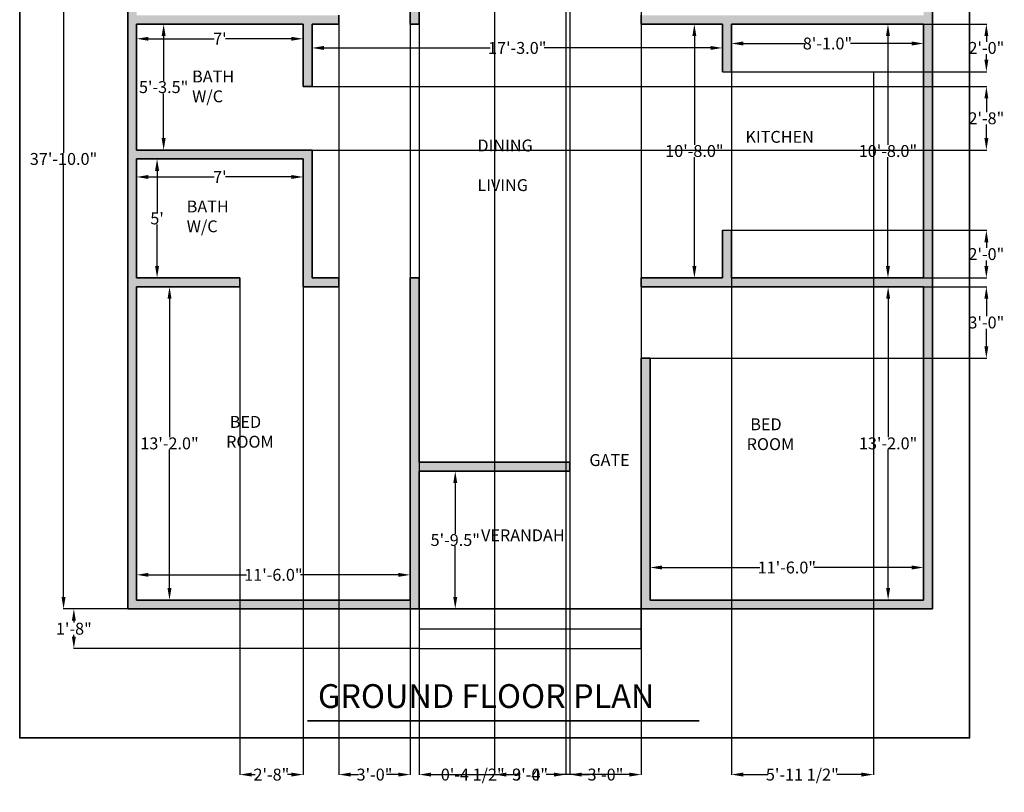
# Model space of a CAD drawing. Units: inches. Extents: x 290 to 786, y 704 to 1301.
# Tile 1 of 2: x 290 to 786, y 704 to 1094. Entities that reach past the tile are written whole.
import ezdxf

# ---------------------------------------------------------------- set-up
doc = ezdxf.new("R2010")
doc.units = ezdxf.units.IN
doc.header["$MEASUREMENT"] = 0
for name, color, linetype, lineweight in [('A-ANNO-DIMS', 2, 'Continuous', 18), ('A-ANNO-TEXT', 7, 'Continuous', 18), ('A-ANNO-TTLB', 7, 'Continuous', 35), ('A-AREA-IDEN', 150, 'Continuous', 25), ('A-FLOR-FIXT', 9, 'Continuous', 25), ('A-FLOR-STRS', 7, 'Continuous', 25), ('A-WALL', 7, 'Continuous', 35)]:
    doc.layers.add(name, color=color, linetype=linetype, lineweight=lineweight)
doc.layers.add('A-WALL-PATT', color=2, linetype='Continuous', lineweight=13, true_color=0xf1eb1f)
doc.styles.get("Standard").update_dxf_attribs({"font": 'arial.ttf'})
doc.dimstyles.get("Standard").update_dxf_attribs({"dimtxt": 6, "dimasz": 6, "dimexe": 0.18, "dimexo": 0.0625, "dimgap": 0.09, "dimtad": 0, "dimtih": 1, "dimtoh": 1, "dimdec": 1, "dimzin": 0, "dimdsep": 46, "dimlunit": 3, "dimtxsty": 'Standard', "dimcen": 0.09, "dimadec": 0, "dimazin": 0, "dimtfac": 1, "dimtdec": 1, "dimtofl": 0, "dimtmove": 0, "dimatfit": 3, "dimfxl": 1, "dimtolj": 1, "dimtzin": 0, "dimarcsym": 0})

# ---------------------------------------------------------------- blocks, each defined once
blk = doc.blocks.new('*D6')
at = {"layer": 'A-ANNO-DIMS', "color": 0, "lineweight": -2, "transparency": 16777216}
for p, q in [((648.53, 1091.27), (648.53, 1081.39)), ((745.53, 1091.27), (745.53, 1081.39)), ((654.53, 1081.57), (685.47, 1081.57)), ((739.53, 1081.57), (708.6, 1081.57))]:
    blk.add_line(p, q, dxfattribs=at)
at = {"layer": 'A-ANNO-DIMS', "color": 0, "transparency": 16777216}
for points in [[(654.53, 1082.57), (654.53, 1080.57), (648.53, 1081.57)], [(739.53, 1082.57), (739.53, 1080.57), (745.53, 1081.57)]]:
    blk.add_solid(points, dxfattribs=at)
at = {"layer": 'Defpoints', "color": 0, "transparency": 16777216}
for p in [(648.53, 1091.33), (745.53, 1091.33), (745.53, 1081.57)]:
    blk.add_point(p, dxfattribs=at)
at = {"layer": 'A-ANNO-DIMS', "color": 0, "transparency": 16777216, "insert": (697.03, 1081.57), "char_height": 6, "attachment_point": 5}
blk.add_mtext('\\A1;8\'-1.0"', dxfattribs=at)
blk = doc.blocks.new('*D7')
at = {"layer": 'A-ANNO-DIMS', "color": 0, "lineweight": -2, "transparency": 16777216}
for p, q in [((745.47, 1091.33), (727.35, 1091.33)), ((727.53, 1085.33), (727.53, 1030.48)), ((727.53, 969.33), (727.53, 1024.18)), ((745.47, 963.33), (727.35, 963.33))]:
    blk.add_line(p, q, dxfattribs=at)
at = {"layer": 'A-ANNO-DIMS', "color": 0, "transparency": 16777216}
for points in [[(726.53, 1085.33), (728.53, 1085.33), (727.53, 1091.33)], [(726.53, 969.33), (728.53, 969.33), (727.53, 963.33)]]:
    blk.add_solid(points, dxfattribs=at)
at = {"layer": 'Defpoints', "color": 0, "transparency": 16777216}
for p in [(745.53, 1091.33), (727.53, 963.33), (745.53, 963.33)]:
    blk.add_point(p, dxfattribs=at)
at = {"layer": 'A-ANNO-DIMS', "color": 0, "transparency": 16777216, "insert": (727.53, 1027.33), "char_height": 6, "attachment_point": 5}
blk.add_mtext('\\A1;10\'-8.0"', dxfattribs=at)
blk = doc.blocks.new('*D8')
at = {"layer": 'A-ANNO-DIMS', "color": 0, "lineweight": -2, "transparency": 16777216}
for p, q in [((607.53, 800.89), (607.53, 817.41)), ((613.53, 817.23), (662.92, 817.23)), ((739.53, 817.23), (690.14, 817.23)), ((745.53, 800.89), (745.53, 817.41))]:
    blk.add_line(p, q, dxfattribs=at)
at = {"layer": 'A-ANNO-DIMS', "color": 0, "transparency": 16777216}
for points in [[(613.53, 818.23), (613.53, 816.23), (607.53, 817.23)], [(739.53, 818.23), (739.53, 816.23), (745.53, 817.23)]]:
    blk.add_solid(points, dxfattribs=at)
at = {"layer": 'Defpoints', "color": 0, "transparency": 16777216}
for p in [(745.53, 817.23), (607.53, 800.83), (745.53, 800.83)]:
    blk.add_point(p, dxfattribs=at)
at = {"layer": 'A-ANNO-DIMS', "color": 0, "transparency": 16777216, "insert": (676.53, 817.23), "char_height": 6, "attachment_point": 5}
blk.add_mtext('\\A1;11\'-6.0"', dxfattribs=at)
blk = doc.blocks.new('*D9')
at = {"layer": 'A-ANNO-DIMS', "color": 0, "lineweight": -2, "transparency": 16777216}
for p, q in [((745.47, 958.83), (727.44, 958.83)), ((727.62, 952.83), (727.62, 882.98)), ((727.62, 806.83), (727.62, 876.67)), ((745.47, 800.83), (727.44, 800.83))]:
    blk.add_line(p, q, dxfattribs=at)
at = {"layer": 'A-ANNO-DIMS', "color": 0, "transparency": 16777216}
for points in [[(726.62, 952.83), (728.62, 952.83), (727.62, 958.83)], [(726.62, 806.83), (728.62, 806.83), (727.62, 800.83)]]:
    blk.add_solid(points, dxfattribs=at)
at = {"layer": 'Defpoints', "color": 0, "transparency": 16777216}
for p in [(745.53, 958.83), (727.62, 800.83), (745.53, 800.83)]:
    blk.add_point(p, dxfattribs=at)
at = {"layer": 'A-ANNO-DIMS', "color": 0, "transparency": 16777216, "insert": (727.62, 879.83), "char_height": 6, "attachment_point": 5}
blk.add_mtext('\\A1;13\'-2.0"', dxfattribs=at)
blk = doc.blocks.new('*D10')
at = {"layer": 'A-ANNO-DIMS', "color": 0, "lineweight": -2, "transparency": 16777216}
for p, q in [((348.6, 958.83), (365.31, 958.83)), ((365.13, 952.83), (365.13, 882.98)), ((365.13, 806.83), (365.13, 876.67)), ((348.6, 800.83), (365.31, 800.83))]:
    blk.add_line(p, q, dxfattribs=at)
at = {"layer": 'A-ANNO-DIMS', "color": 0, "transparency": 16777216}
for points in [[(364.13, 952.83), (366.13, 952.83), (365.13, 958.83)], [(364.13, 806.83), (366.13, 806.83), (365.13, 800.83)]]:
    blk.add_solid(points, dxfattribs=at)
at = {"layer": 'Defpoints', "color": 0, "transparency": 16777216}
for p in [(348.53, 958.83), (348.53, 800.83), (365.13, 800.83)]:
    blk.add_point(p, dxfattribs=at)
at = {"layer": 'A-ANNO-DIMS', "color": 0, "transparency": 16777216, "insert": (365.13, 879.83), "char_height": 6, "attachment_point": 5}
blk.add_mtext('\\A1;13\'-2.0"', dxfattribs=at)
blk = doc.blocks.new('*D11')
at = {"layer": 'A-ANNO-DIMS', "color": 0, "lineweight": -2, "transparency": 16777216}
for p, q in [((348.53, 800.89), (348.53, 813.7)), ((354.53, 813.52), (403.92, 813.52)), ((480.53, 813.52), (431.14, 813.52)), ((486.53, 800.89), (486.53, 813.7))]:
    blk.add_line(p, q, dxfattribs=at)
at = {"layer": 'A-ANNO-DIMS', "color": 0, "transparency": 16777216}
for points in [[(354.53, 814.52), (354.53, 812.52), (348.53, 813.52)], [(480.53, 814.52), (480.53, 812.52), (486.53, 813.52)]]:
    blk.add_solid(points, dxfattribs=at)
at = {"layer": 'Defpoints', "color": 0, "transparency": 16777216}
for p in [(486.53, 813.52), (348.53, 800.83), (486.53, 800.83)]:
    blk.add_point(p, dxfattribs=at)
at = {"layer": 'A-ANNO-DIMS', "color": 0, "transparency": 16777216, "insert": (417.53, 813.52), "char_height": 6, "attachment_point": 5}
blk.add_mtext('\\A1;11\'-6.0"', dxfattribs=at)
blk = doc.blocks.new('*D12')
at = {"layer": 'A-ANNO-DIMS', "color": 0, "lineweight": -2, "transparency": 16777216}
for p, q in [((348.6, 1091.33), (362.35, 1091.33)), ((362.17, 1085.33), (362.17, 1062.73)), ((362.17, 1033.83), (362.17, 1056.42)), ((348.6, 1027.83), (362.35, 1027.83))]:
    blk.add_line(p, q, dxfattribs=at)
at = {"layer": 'A-ANNO-DIMS', "color": 0, "transparency": 16777216}
for points in [[(361.17, 1085.33), (363.17, 1085.33), (362.17, 1091.33)], [(361.17, 1033.83), (363.17, 1033.83), (362.17, 1027.83)]]:
    blk.add_solid(points, dxfattribs=at)
at = {"layer": 'Defpoints', "color": 0, "transparency": 16777216}
for p in [(348.53, 1091.33), (348.53, 1027.83), (362.17, 1027.83)]:
    blk.add_point(p, dxfattribs=at)
at = {"layer": 'A-ANNO-DIMS', "color": 0, "transparency": 16777216, "insert": (362.17, 1059.58), "char_height": 6, "attachment_point": 5}
blk.add_mtext('\\A1;5\'-3.5"', dxfattribs=at)
blk = doc.blocks.new('*D13')
at = {"layer": 'A-ANNO-DIMS', "color": 0, "lineweight": -2, "transparency": 16777216}
for p, q in [((348.53, 1091.27), (348.53, 1083.77)), ((432.53, 1091.27), (432.53, 1083.77)), ((354.53, 1083.95), (387.71, 1083.95)), ((426.53, 1083.95), (393.36, 1083.95))]:
    blk.add_line(p, q, dxfattribs=at)
at = {"layer": 'A-ANNO-DIMS', "color": 0, "transparency": 16777216}
for points in [[(354.53, 1084.95), (354.53, 1082.95), (348.53, 1083.95)], [(426.53, 1084.95), (426.53, 1082.95), (432.53, 1083.95)]]:
    blk.add_solid(points, dxfattribs=at)
at = {"layer": 'Defpoints', "color": 0, "transparency": 16777216}
for p in [(348.53, 1091.33), (432.53, 1091.33), (432.53, 1083.95)]:
    blk.add_point(p, dxfattribs=at)
at = {"layer": 'A-ANNO-DIMS', "color": 0, "transparency": 16777216, "insert": (390.53, 1083.95), "char_height": 6, "attachment_point": 5}
blk.add_mtext("\\A1;7'", dxfattribs=at)
blk = doc.blocks.new('*D14')
at = {"layer": 'A-ANNO-DIMS', "color": 0, "lineweight": -2, "transparency": 16777216}
for p, q in [((348.6, 1023.33), (359.04, 1023.33)), ((358.86, 1017.33), (358.86, 996.47)), ((358.86, 969.33), (358.86, 990.19)), ((348.6, 963.33), (359.04, 963.33))]:
    blk.add_line(p, q, dxfattribs=at)
at = {"layer": 'A-ANNO-DIMS', "color": 0, "transparency": 16777216}
for points in [[(357.86, 1017.33), (359.86, 1017.33), (358.86, 1023.33)], [(357.86, 969.33), (359.86, 969.33), (358.86, 963.33)]]:
    blk.add_solid(points, dxfattribs=at)
at = {"layer": 'Defpoints', "color": 0, "transparency": 16777216}
for p in [(348.53, 1023.33), (358.86, 1023.33), (348.53, 963.33)]:
    blk.add_point(p, dxfattribs=at)
at = {"layer": 'A-ANNO-DIMS', "color": 0, "transparency": 16777216, "insert": (358.86, 993.33), "char_height": 6, "attachment_point": 5}
blk.add_mtext("\\A1;5'", dxfattribs=at)
blk = doc.blocks.new('*D15')
at = {"layer": 'A-ANNO-DIMS', "color": 0, "lineweight": -2, "transparency": 16777216}
for p, q in [((348.53, 1023.27), (348.53, 1014.06)), ((432.53, 1023.27), (432.53, 1014.06)), ((354.53, 1014.24), (387.71, 1014.24)), ((426.53, 1014.24), (393.36, 1014.24))]:
    blk.add_line(p, q, dxfattribs=at)
at = {"layer": 'A-ANNO-DIMS', "color": 0, "transparency": 16777216}
for points in [[(354.53, 1015.24), (354.53, 1013.24), (348.53, 1014.24)], [(426.53, 1015.24), (426.53, 1013.24), (432.53, 1014.24)]]:
    blk.add_solid(points, dxfattribs=at)
at = {"layer": 'Defpoints', "color": 0, "transparency": 16777216}
for p in [(348.53, 1023.33), (432.53, 1023.33), (432.53, 1014.24)]:
    blk.add_point(p, dxfattribs=at)
at = {"layer": 'A-ANNO-DIMS', "color": 0, "transparency": 16777216, "insert": (390.53, 1014.24), "char_height": 6, "attachment_point": 5}
blk.add_mtext("\\A1;7'", dxfattribs=at)
blk = doc.blocks.new('*D16')
at = {"layer": 'A-ANNO-DIMS', "color": 0, "lineweight": -2, "transparency": 16777216}
for p, q in [((491.1, 865.83), (509.45, 865.83)), ((509.27, 859.83), (509.27, 834.23)), ((509.27, 802.33), (509.27, 827.93)), ((491.1, 796.33), (509.45, 796.33))]:
    blk.add_line(p, q, dxfattribs=at)
at = {"layer": 'A-ANNO-DIMS', "color": 0, "transparency": 16777216}
for points in [[(508.27, 859.83), (510.27, 859.83), (509.27, 865.83)], [(508.27, 802.33), (510.27, 802.33), (509.27, 796.33)]]:
    blk.add_solid(points, dxfattribs=at)
at = {"layer": 'Defpoints', "color": 0, "transparency": 16777216}
for p in [(491.03, 865.83), (509.27, 865.83), (491.03, 796.33)]:
    blk.add_point(p, dxfattribs=at)
at = {"layer": 'A-ANNO-DIMS', "color": 0, "transparency": 16777216, "insert": (509.27, 831.08), "char_height": 6, "width": 22.94, "attachment_point": 5}
blk.add_mtext('\\A1;5\'-9.5"', dxfattribs=at)
blk = doc.blocks.new('*D18')
at = {"layer": 'A-ANNO-DIMS', "color": 0, "lineweight": -2, "transparency": 16777216}
for p, q in [((343.97, 1250.33), (311.5, 1250.33)), ((311.68, 1244.33), (311.68, 1026.48)), ((311.68, 802.33), (311.68, 1020.17)), ((343.97, 796.33), (311.5, 796.33))]:
    blk.add_line(p, q, dxfattribs=at)
at = {"layer": 'A-ANNO-DIMS', "color": 0, "transparency": 16777216}
for points in [[(310.68, 1244.33), (312.68, 1244.33), (311.68, 1250.33)], [(310.68, 802.33), (312.68, 802.33), (311.68, 796.33)]]:
    blk.add_solid(points, dxfattribs=at)
at = {"layer": 'Defpoints', "color": 0, "transparency": 16777216}
for p in [(344.03, 1250.33), (311.68, 796.33), (344.03, 796.33)]:
    blk.add_point(p, dxfattribs=at)
at = {"layer": 'A-ANNO-DIMS', "color": 0, "transparency": 16777216, "insert": (311.68, 1023.33), "char_height": 6, "attachment_point": 5}
blk.add_mtext('\\A1;37\'-10.0"', dxfattribs=at)
blk = doc.blocks.new('*D19')
at = {"layer": 'A-ANNO-DIMS', "color": 0, "lineweight": -2, "transparency": 16777216}
for p, q in [((629.96, 1091.33), (630.07, 1091.33)), ((629.89, 1085.33), (629.89, 1030.48)), ((629.89, 969.33), (629.89, 1024.18)), ((629.96, 963.33), (630.07, 963.33))]:
    blk.add_line(p, q, dxfattribs=at)
at = {"layer": 'A-ANNO-DIMS', "color": 0, "transparency": 16777216}
for points in [[(628.89, 1085.33), (630.89, 1085.33), (629.89, 1091.33)], [(628.89, 969.33), (630.89, 969.33), (629.89, 963.33)]]:
    blk.add_solid(points, dxfattribs=at)
at = {"layer": 'Defpoints', "color": 0, "transparency": 16777216}
for p in [(629.89, 1091.33), (629.89, 963.33), (629.89, 963.33)]:
    blk.add_point(p, dxfattribs=at)
at = {"layer": 'A-ANNO-DIMS', "color": 0, "transparency": 16777216, "insert": (629.89, 1027.33), "char_height": 6, "attachment_point": 5}
blk.add_mtext('\\A1;10\'-8.0"', dxfattribs=at)
blk = doc.blocks.new('*D20')
at = {"layer": 'A-ANNO-DIMS', "color": 0, "lineweight": -2, "transparency": 16777216}
for p, q in [((437.03, 1091.27), (437.03, 1079.15)), ((644.03, 1091.27), (644.03, 1079.15)), ((443.03, 1079.33), (526.92, 1079.33)), ((638.03, 1079.33), (554.14, 1079.33))]:
    blk.add_line(p, q, dxfattribs=at)
at = {"layer": 'A-ANNO-DIMS', "color": 0, "transparency": 16777216}
for points in [[(443.03, 1080.33), (443.03, 1078.33), (437.03, 1079.33)], [(638.03, 1080.33), (638.03, 1078.33), (644.03, 1079.33)]]:
    blk.add_solid(points, dxfattribs=at)
at = {"layer": 'Defpoints', "color": 0, "transparency": 16777216}
for p in [(437.03, 1091.33), (644.03, 1091.33), (644.03, 1079.33)]:
    blk.add_point(p, dxfattribs=at)
at = {"layer": 'A-ANNO-DIMS', "color": 0, "transparency": 16777216, "insert": (540.53, 1079.33), "char_height": 6, "attachment_point": 5}
blk.add_mtext('\\A1;17\'-3.0"', dxfattribs=at)
blk = doc.blocks.new('*D22')
at = {"layer": 'A-ANNO-DIMS', "color": 0, "lineweight": -2, "transparency": 16777216}
for p, q in [((567.03, 1149.77), (567.03, 712.58)), ((603.03, 1149.77), (603.03, 712.58)), ((573.03, 712.76), (576.97, 712.76)), ((597.03, 712.76), (593.1, 712.76))]:
    blk.add_line(p, q, dxfattribs=at)
at = {"layer": 'A-ANNO-DIMS', "color": 0, "transparency": 16777216}
for points in [[(573.03, 713.76), (573.03, 711.76), (567.03, 712.76)], [(597.03, 713.76), (597.03, 711.76), (603.03, 712.76)]]:
    blk.add_solid(points, dxfattribs=at)
at = {"layer": 'Defpoints', "color": 0, "transparency": 16777216}
for p in [(567.03, 1149.83), (603.03, 1149.83), (603.03, 712.76)]:
    blk.add_point(p, dxfattribs=at)
at = {"layer": 'A-ANNO-DIMS', "color": 0, "transparency": 16777216, "insert": (585.03, 712.76), "char_height": 6, "attachment_point": 5}
blk.add_mtext('\\A1;3\'-0"', dxfattribs=at)
blk = doc.blocks.new('*D24')
at = {"layer": 'A-ANNO-DIMS', "color": 0, "lineweight": -2, "transparency": 16777216}
for p, q in [((529.03, 1149.77), (529.03, 712.58)), ((565.03, 1149.77), (565.03, 712.58)), ((535.03, 712.76), (538.97, 712.76)), ((559.03, 712.76), (555.1, 712.76))]:
    blk.add_line(p, q, dxfattribs=at)
at = {"layer": 'A-ANNO-DIMS', "color": 0, "transparency": 16777216}
for points in [[(535.03, 713.76), (535.03, 711.76), (529.03, 712.76)], [(559.03, 713.76), (559.03, 711.76), (565.03, 712.76)]]:
    blk.add_solid(points, dxfattribs=at)
at = {"layer": 'Defpoints', "color": 0, "transparency": 16777216}
for p in [(529.03, 1149.83), (565.03, 1149.83), (565.03, 712.76)]:
    blk.add_point(p, dxfattribs=at)
at = {"layer": 'A-ANNO-DIMS', "color": 0, "transparency": 16777216, "insert": (547.03, 712.76), "char_height": 6, "attachment_point": 5}
blk.add_mtext('\\A1;3\'-0"', dxfattribs=at)
blk = doc.blocks.new('*D26')
at = {"layer": 'A-ANNO-DIMS', "color": 0, "lineweight": -2, "transparency": 16777216}
for p, q in [((491.03, 776.27), (491.03, 712.58)), ((603.03, 776.27), (603.03, 712.58)), ((497.03, 712.76), (538.97, 712.76)), ((597.03, 712.76), (555.1, 712.76))]:
    blk.add_line(p, q, dxfattribs=at)
at = {"layer": 'A-ANNO-DIMS', "color": 0, "transparency": 16777216}
for points in [[(497.03, 713.76), (497.03, 711.76), (491.03, 712.76)], [(597.03, 713.76), (597.03, 711.76), (603.03, 712.76)]]:
    blk.add_solid(points, dxfattribs=at)
at = {"layer": 'Defpoints', "color": 0, "transparency": 16777216}
for p in [(491.03, 776.33), (603.03, 776.33), (603.03, 712.76)]:
    blk.add_point(p, dxfattribs=at)
at = {"layer": 'A-ANNO-DIMS', "color": 0, "transparency": 16777216, "insert": (547.03, 712.76), "char_height": 6, "attachment_point": 5}
blk.add_mtext('\\A1;9\'-4"', dxfattribs=at)
blk = doc.blocks.new('*D27')
at = {"layer": 'A-ANNO-DIMS', "color": 0, "lineweight": -2, "transparency": 16777216}
for p, q in [((490.97, 796.33), (316.7, 796.33)), ((316.88, 790.33), (316.88, 789.48)), ((316.88, 782.33), (316.88, 783.18)), ((490.97, 776.33), (316.7, 776.33))]:
    blk.add_line(p, q, dxfattribs=at)
at = {"layer": 'A-ANNO-DIMS', "color": 0, "transparency": 16777216}
for points in [[(315.88, 790.33), (317.88, 790.33), (316.88, 796.33)], [(315.88, 782.33), (317.88, 782.33), (316.88, 776.33)]]:
    blk.add_solid(points, dxfattribs=at)
at = {"layer": 'Defpoints', "color": 0, "transparency": 16777216}
for p in [(316.88, 796.33), (491.03, 796.33), (491.03, 776.33)]:
    blk.add_point(p, dxfattribs=at)
at = {"layer": 'A-ANNO-DIMS', "color": 0, "transparency": 16777216, "insert": (316.88, 786.33), "char_height": 6, "attachment_point": 5}
blk.add_mtext('\\A1;1\'-8"', dxfattribs=at)
blk = doc.blocks.new('*D28')
at = {"layer": 'A-ANNO-DIMS', "color": 0, "lineweight": -2, "transparency": 16777216}
for p, q in [((603.03, 922.77), (603.03, 712.58)), ((567.03, 865.77), (567.03, 712.58)), ((573.03, 712.76), (576.97, 712.76)), ((597.03, 712.76), (593.1, 712.76))]:
    blk.add_line(p, q, dxfattribs=at)
at = {"layer": 'A-ANNO-DIMS', "color": 0, "transparency": 16777216}
for points in [[(573.03, 713.76), (573.03, 711.76), (567.03, 712.76)], [(597.03, 713.76), (597.03, 711.76), (603.03, 712.76)]]:
    blk.add_solid(points, dxfattribs=at)
at = {"layer": 'Defpoints', "color": 0, "transparency": 16777216}
for p in [(603.03, 922.83), (567.03, 865.83), (603.03, 712.76)]:
    blk.add_point(p, dxfattribs=at)
at = {"layer": 'A-ANNO-DIMS', "color": 0, "transparency": 16777216, "insert": (585.03, 712.76), "char_height": 6, "attachment_point": 5}
blk.add_mtext('\\A1;3\'-0"', dxfattribs=at)
blk = doc.blocks.new('*D29')
at = {"layer": 'A-ANNO-DIMS', "color": 0, "lineweight": -2, "transparency": 16777216}
for p, q in [((400.53, 958.77), (400.53, 712.58)), ((432.53, 958.77), (432.53, 712.58)), ((406.53, 712.76), (408.42, 712.76)), ((426.53, 712.76), (424.65, 712.76))]:
    blk.add_line(p, q, dxfattribs=at)
at = {"layer": 'A-ANNO-DIMS', "color": 0, "transparency": 16777216}
for points in [[(406.53, 713.76), (406.53, 711.76), (400.53, 712.76)], [(426.53, 713.76), (426.53, 711.76), (432.53, 712.76)]]:
    blk.add_solid(points, dxfattribs=at)
at = {"layer": 'Defpoints', "color": 0, "transparency": 16777216}
for p in [(400.53, 958.83), (432.53, 958.83), (432.53, 712.76)]:
    blk.add_point(p, dxfattribs=at)
at = {"layer": 'A-ANNO-DIMS', "color": 0, "transparency": 16777216, "insert": (416.53, 712.76), "char_height": 6, "attachment_point": 5}
blk.add_mtext('\\A1;2\'-8"', dxfattribs=at)
blk = doc.blocks.new('*D30')
at = {"layer": 'A-ANNO-DIMS', "color": 0, "lineweight": -2, "transparency": 16777216}
for p, q in [((437.1, 1059.83), (777.36, 1059.83)), ((777.18, 1053.83), (777.18, 1046.98)), ((777.18, 1033.83), (777.18, 1040.68)), ((437.1, 1027.83), (777.36, 1027.83))]:
    blk.add_line(p, q, dxfattribs=at)
at = {"layer": 'A-ANNO-DIMS', "color": 0, "transparency": 16777216}
for points in [[(776.18, 1053.83), (778.18, 1053.83), (777.18, 1059.83)], [(776.18, 1033.83), (778.18, 1033.83), (777.18, 1027.83)]]:
    blk.add_solid(points, dxfattribs=at)
at = {"layer": 'Defpoints', "color": 0, "transparency": 16777216}
for p in [(437.03, 1059.83), (777.18, 1059.83), (437.03, 1027.83)]:
    blk.add_point(p, dxfattribs=at)
at = {"layer": 'A-ANNO-DIMS', "color": 0, "transparency": 16777216, "insert": (777.18, 1043.83), "char_height": 6, "attachment_point": 5}
blk.add_mtext('\\A1;2\'-8"', dxfattribs=at)
blk = doc.blocks.new('*D31')
at = {"layer": 'A-ANNO-DIMS', "color": 0, "lineweight": -2, "transparency": 16777216}
for p, q in [((450.53, 958.77), (450.53, 712.58)), ((486.53, 963.27), (486.53, 712.58)), ((456.53, 712.76), (460.47, 712.76)), ((480.53, 712.76), (476.6, 712.76))]:
    blk.add_line(p, q, dxfattribs=at)
at = {"layer": 'A-ANNO-DIMS', "color": 0, "transparency": 16777216}
for points in [[(456.53, 713.76), (456.53, 711.76), (450.53, 712.76)], [(480.53, 713.76), (480.53, 711.76), (486.53, 712.76)]]:
    blk.add_solid(points, dxfattribs=at)
at = {"layer": 'Defpoints', "color": 0, "transparency": 16777216}
for p in [(450.53, 958.83), (486.53, 963.33), (486.53, 712.76)]:
    blk.add_point(p, dxfattribs=at)
at = {"layer": 'A-ANNO-DIMS', "color": 0, "transparency": 16777216, "insert": (468.53, 712.76), "char_height": 6, "attachment_point": 5}
blk.add_mtext('\\A1;3\'-0"', dxfattribs=at)
blk = doc.blocks.new('*D32')
at = {"layer": 'A-ANNO-DIMS', "color": 0, "lineweight": -2, "transparency": 16777216}
for p, q in [((603.1, 958.83), (777.36, 958.83)), ((777.18, 952.83), (777.18, 943.98)), ((777.18, 928.83), (777.18, 937.67)), ((607.6, 922.83), (777.36, 922.83))]:
    blk.add_line(p, q, dxfattribs=at)
at = {"layer": 'A-ANNO-DIMS', "color": 0, "transparency": 16777216}
for points in [[(776.18, 952.83), (778.18, 952.83), (777.18, 958.83)], [(776.18, 928.83), (778.18, 928.83), (777.18, 922.83)]]:
    blk.add_solid(points, dxfattribs=at)
at = {"layer": 'Defpoints', "color": 0, "transparency": 16777216}
for p in [(603.03, 958.83), (607.53, 922.83), (777.18, 922.83)]:
    blk.add_point(p, dxfattribs=at)
at = {"layer": 'A-ANNO-DIMS', "color": 0, "transparency": 16777216, "insert": (777.18, 940.83), "char_height": 6, "attachment_point": 5}
blk.add_mtext('\\A1;3\'-0"', dxfattribs=at)
blk = doc.blocks.new('*D33')
at = {"layer": 'A-ANNO-DIMS', "color": 0, "lineweight": -2, "transparency": 16777216}
for p, q in [((450.53, 1091.27), (450.53, 712.58)), ((486.53, 1091.27), (486.53, 712.58)), ((456.53, 712.76), (460.47, 712.76)), ((480.53, 712.76), (476.6, 712.76))]:
    blk.add_line(p, q, dxfattribs=at)
at = {"layer": 'A-ANNO-DIMS', "color": 0, "transparency": 16777216}
for points in [[(456.53, 713.76), (456.53, 711.76), (450.53, 712.76)], [(480.53, 713.76), (480.53, 711.76), (486.53, 712.76)]]:
    blk.add_solid(points, dxfattribs=at)
at = {"layer": 'Defpoints', "color": 0, "transparency": 16777216}
for p in [(450.53, 1091.33), (486.53, 1091.33), (486.53, 712.76)]:
    blk.add_point(p, dxfattribs=at)
at = {"layer": 'A-ANNO-DIMS', "color": 0, "transparency": 16777216, "insert": (468.53, 712.76), "char_height": 6, "attachment_point": 5}
blk.add_mtext('\\A1;3\'-0"', dxfattribs=at)
blk = doc.blocks.new('*D35')
at = {"layer": 'A-ANNO-DIMS', "color": 0, "lineweight": -2, "transparency": 16777216}
for p, q in [((648.6, 1091.33), (777.36, 1091.33)), ((777.18, 1085.33), (777.18, 1082.48)), ((777.18, 1073.33), (777.18, 1076.18)), ((648.6, 1067.33), (777.36, 1067.33))]:
    blk.add_line(p, q, dxfattribs=at)
at = {"layer": 'A-ANNO-DIMS', "color": 0, "transparency": 16777216}
for points in [[(776.18, 1085.33), (778.18, 1085.33), (777.18, 1091.33)], [(776.18, 1073.33), (778.18, 1073.33), (777.18, 1067.33)]]:
    blk.add_solid(points, dxfattribs=at)
at = {"layer": 'Defpoints', "color": 0, "transparency": 16777216}
for p in [(648.53, 1091.33), (648.53, 1067.33), (777.18, 1067.33)]:
    blk.add_point(p, dxfattribs=at)
at = {"layer": 'A-ANNO-DIMS', "color": 0, "transparency": 16777216, "insert": (777.18, 1079.33), "char_height": 6, "attachment_point": 5}
blk.add_mtext('\\A1;2\'-0"', dxfattribs=at)
blk = doc.blocks.new('*D36')
at = {"layer": 'A-ANNO-DIMS', "color": 0, "lineweight": -2, "transparency": 16777216}
for p, q in [((648.53, 1067.27), (648.53, 712.58)), ((720.17, 1067.27), (720.17, 712.58)), ((654.53, 712.76), (666.97, 712.76)), ((714.17, 712.76), (701.74, 712.76))]:
    blk.add_line(p, q, dxfattribs=at)
at = {"layer": 'A-ANNO-DIMS', "color": 0, "transparency": 16777216}
for points in [[(654.53, 713.76), (654.53, 711.76), (648.53, 712.76)], [(714.17, 713.76), (714.17, 711.76), (720.17, 712.76)]]:
    blk.add_solid(points, dxfattribs=at)
at = {"layer": 'Defpoints', "color": 0, "transparency": 16777216}
for p in [(648.53, 1067.33), (720.17, 1067.33), (720.17, 712.76)]:
    blk.add_point(p, dxfattribs=at)
at = {"layer": 'A-ANNO-DIMS', "color": 0, "transparency": 16777216, "insert": (684.35, 712.76), "char_height": 6, "attachment_point": 5}
blk.add_mtext('\\A1;5\'-11 1/2"', dxfattribs=at)
blk = doc.blocks.new('*D37')
at = {"layer": 'A-ANNO-DIMS', "color": 0, "lineweight": -2, "transparency": 16777216}
for p, q in [((648.6, 987.33), (777.36, 987.33)), ((777.18, 981.33), (777.18, 978.48)), ((777.18, 969.33), (777.18, 972.18)), ((648.6, 963.33), (777.36, 963.33))]:
    blk.add_line(p, q, dxfattribs=at)
at = {"layer": 'A-ANNO-DIMS', "color": 0, "transparency": 16777216}
for points in [[(776.18, 981.33), (778.18, 981.33), (777.18, 987.33)], [(776.18, 969.33), (778.18, 969.33), (777.18, 963.33)]]:
    blk.add_solid(points, dxfattribs=at)
at = {"layer": 'Defpoints', "color": 0, "transparency": 16777216}
for p in [(648.53, 987.33), (777.18, 987.33), (648.53, 963.33)]:
    blk.add_point(p, dxfattribs=at)
at = {"layer": 'A-ANNO-DIMS', "color": 0, "transparency": 16777216, "insert": (777.18, 975.33), "char_height": 6, "attachment_point": 5}
blk.add_mtext('\\A1;2\'-0"', dxfattribs=at)
blk = doc.blocks.new('*D38')
at = {"layer": 'A-ANNO-DIMS', "color": 0, "lineweight": -2, "transparency": 16777216}
for p, q in [((486.53, 1091.27), (486.53, 712.58)), ((491.03, 1091.27), (491.03, 712.58)), ((480.53, 712.76), (474.53, 712.76)), ((497.03, 712.76), (503.03, 712.76))]:
    blk.add_line(p, q, dxfattribs=at)
at = {"layer": 'A-ANNO-DIMS', "color": 0, "transparency": 16777216}
for points in [[(480.53, 713.76), (480.53, 711.76), (486.53, 712.76)], [(497.03, 713.76), (497.03, 711.76), (491.03, 712.76)]]:
    blk.add_solid(points, dxfattribs=at)
at = {"layer": 'Defpoints', "color": 0, "transparency": 16777216}
for p in [(486.53, 1091.33), (491.03, 1091.33), (491.03, 712.76)]:
    blk.add_point(p, dxfattribs=at)
at = {"layer": 'A-ANNO-DIMS', "color": 0, "transparency": 16777216, "insert": (518.09, 712.76), "char_height": 6, "attachment_point": 5}
blk.add_mtext('\\A1;0\'-4 1/2"', dxfattribs=at)

msp = doc.modelspace()

# ---------------------------------------------------------------- hatches: boundary and pattern name
at = {"layer": 'A-WALL-PATT'}
h = msp.add_hatch(color=256, dxfattribs=at)
h.dxf.hatch_style = 1
h.paths.add_polyline_path([(750.03, 1250.33), (344.03, 1250.33), (344.03, 796.33), (491.03, 796.33), (491.03, 865.83), (567.03, 865.83), (567.03, 870.33), (491.03, 870.33), (491.03, 963.33), (486.53, 963.33), (486.53, 800.83), (348.53, 800.83), (348.53, 958.83), (400.53, 958.83), (400.53, 963.33), (348.53, 963.33), (348.53, 1023.33), (432.53, 1023.33), (432.53, 958.83), (450.53, 958.83), (450.53, 963.33), (437.03, 963.33), (437.03, 1027.83), (348.53, 1027.83), (348.53, 1091.33), (432.53, 1091.33), (432.53, 1059.83), (437.03, 1059.83), (437.03, 1091.33), (450.53, 1091.33), (450.53, 1095.83), (348.53, 1095.83), (348.53, 1245.83), (486.53, 1245.83), (486.53, 1091.33), (491.03, 1091.33), (491.03, 1245.83), (603.03, 1245.83), (603.03, 1131.83), (607.53, 1131.83), (607.53, 1245.83), (745.53, 1245.83), (745.53, 1095.83), (603.03, 1095.83), (603.03, 1091.33), (644.03, 1091.33), (644.03, 1067.33), (648.53, 1067.33), (648.53, 1091.33), (745.53, 1091.33), (745.53, 963.33), (648.53, 963.33), (648.53, 987.33), (644.03, 987.33), (644.03, 963.33), (603.03, 963.33), (603.03, 958.83), (745.53, 958.83), (745.53, 800.83), (607.53, 800.83), (607.53, 922.83), (603.03, 922.83), (603.03, 796.33), (750.03, 796.33)])

# ---------------------------------------------------------------- linework, layer by layer
at = {"layer": 'A-ANNO-TTLB'}
for p, q in [((434.67, 739.91), (627.58, 739.91)), ((627.58, 739.91), (632.31, 739.91))]:
    msp.add_line(p, q, dxfattribs=at)
msp.add_lwpolyline([(289.56, 1300.6), (768.7, 1300.6), (768.7, 731.29), (289.56, 731.29)], close=True, dxfattribs=at)
at = {"layer": 'A-FLOR-FIXT'}
for p, q in [((644.03, 1067.33), (720.17, 1067.33)), ((720.17, 1067.33), (720.17, 987.33)), ((644.03, 987.33), (720.17, 987.33))]:
    msp.add_line(p, q, dxfattribs=at)
at = {"layer": 'A-FLOR-STRS'}
for p, q in [((491.03, 796.33), (491.03, 776.33)), ((603.03, 776.33), (603.03, 796.33)), ((491.03, 786.33), (603.03, 786.33)), ((491.03, 776.33), (603.03, 776.33))]:
    msp.add_line(p, q, dxfattribs=at)
at = {"layer": 'A-WALL'}
for p, q in [((344.03, 1250.33), (344.03, 796.33)), ((750.03, 1250.33), (750.03, 796.33)), ((486.53, 1245.83), (486.53, 1091.33)), ((491.03, 1245.83), (491.03, 1091.33)), ((450.53, 1091.33), (450.53, 1095.83)), ((603.03, 1095.83), (603.03, 1091.33)), ((348.53, 1091.33), (432.53, 1091.33)), ((348.53, 1091.33), (348.53, 1027.83)), ((432.53, 1091.33), (432.53, 1059.83)), ((437.03, 1091.33), (437.03, 1059.83)), ((437.03, 1091.33), (450.53, 1091.33)), ((486.53, 1091.33), (491.03, 1091.33)), ((603.03, 1091.33), (644.03, 1091.33)), ((644.03, 1091.33), (644.03, 1067.33)), ((648.53, 1091.33), (648.53, 1067.33)), ((648.53, 1091.33), (648.53, 1067.33)), ((648.53, 1091.33), (745.53, 1091.33)), ((745.53, 1091.33), (745.53, 963.33)), ((432.53, 1059.83), (437.03, 1059.83)), ((348.53, 1027.83), (437.03, 1027.83)), ((348.53, 1023.33), (432.53, 1023.33)), ((348.53, 1023.33), (348.53, 963.33)), ((432.53, 1023.33), (432.53, 958.83)), ((437.03, 1027.83), (437.03, 963.33)), ((644.03, 987.33), (644.03, 963.33)), ((648.53, 963.33), (648.53, 987.33)), ((648.53, 987.33), (648.53, 963.33)), ((348.53, 963.33), (400.53, 963.33)), ((348.53, 958.83), (400.53, 958.83)), ((348.53, 958.83), (348.53, 800.83)), ((400.53, 963.33), (400.53, 958.83)), ((432.53, 958.83), (450.53, 958.83)), ((437.03, 963.33), (450.53, 963.33)), ((450.53, 963.33), (450.53, 958.83)), ((486.53, 963.33), (486.53, 800.83)), ((486.53, 963.33), (491.03, 963.33)), ((491.03, 963.33), (491.03, 870.33)), ((603.03, 963.33), (644.03, 963.33)), ((603.03, 963.33), (603.03, 958.83)), ((603.03, 958.83), (745.53, 958.83)), ((648.53, 963.33), (745.53, 963.33)), ((745.53, 958.83), (745.53, 800.83)), ((603.03, 922.83), (607.53, 922.83)), ((603.03, 922.83), (603.03, 796.33)), ((607.53, 922.83), (607.53, 800.83)), ((491.03, 870.33), (567.03, 870.33)), ((567.03, 865.83), (567.03, 870.33)), ((491.03, 865.83), (567.03, 865.83)), ((491.03, 865.83), (491.03, 796.33)), ((348.53, 800.83), (486.53, 800.83)), ((607.53, 800.83), (745.53, 800.83)), ((344.03, 796.33), (750.03, 796.33))]:
    msp.add_line(p, q, dxfattribs=at)

# ---------------------------------------------------------------- texts
at = {"layer": 'A-ANNO-TEXT', "insert": (576.93, 874.42), "char_height": 6, "attachment_point": 1}
msp.add_mtext_dynamic_manual_height_columns('GATE', width=21.2425, gutter_width=30, heights=[0], dxfattribs=at)
at = {"layer": 'A-ANNO-TTLB', "insert": (440, 758.37), "char_height": 12, "attachment_point": 1}
msp.add_mtext_dynamic_manual_height_columns('GROUND FLOOR PLAN', width=230.1331, gutter_width=60, heights=[0], dxfattribs=at)
at = {"layer": 'A-AREA-IDEN', "char_height": 6, "attachment_point": 1}
for s, width, insert in [('BATH\\PW/C', 49.7176, (376.53, 1067.92)), ('DINING\\P\\PLIVING', 66.1278, (520.44, 1033.13)), ('KITCHEN', 49.9801, (655.65, 1037.48)), ('BATH\\PW/C', 33.3903, (373.8, 1002.34)), (' BED\\PROOM', 38.2318, (393.69, 893.68)), (' BED\\PROOM', 42.9072, (656.26, 892.46)), ('VERANDAH', 36.2763, (522.28, 836.45))]:
    msp.add_mtext_dynamic_manual_height_columns(s, width=width, gutter_width=30, heights=[0], dxfattribs=dict(at, insert=insert))

# ---------------------------------------------------------------- dimensions: what is measured, and where the dimension line sits
at = {"layer": 'A-ANNO-DIMS'}
for base, p1, p2, override, picture, middle in [((311.68, 796.33), (344.03, 1250.33), (344.03, 796.33), {"dimclrd": 0, "dimclre": 0, "dimclrt": 0}, '*D18', (311.68, 1023.33)), ((362.17, 1027.83), (348.53, 1091.33), (348.53, 1027.83), {"dimclrd": 0, "dimclre": 0, "dimclrt": 0}, '*D12', (362.17, 1059.58)), ((629.89, 963.33), (629.89, 1091.33), (629.89, 963.33), {"dimclrd": 0, "dimclre": 0, "dimclrt": 0}, '*D19', (629.89, 1027.33)), ((777.18, 1067.33), (648.53, 1091.33), (648.53, 1067.33), {"dimdec": 1, "dimlfac": 1, "dimrnd": 0, "dimzin": 1, "dimdsep": 46, "dimlunit": 4, "dimfrac": 2}, '*D35', (777.18, 1079.33)), ((727.53, 963.33), (745.53, 1091.33), (745.53, 963.33), {"dimclrd": 0, "dimclre": 0, "dimclrt": 0}, '*D7', (727.53, 1027.33)), ((777.18, 1059.83), (437.03, 1027.83), (437.03, 1059.83), {"dimdec": 1, "dimlfac": 1, "dimrnd": 0, "dimzin": 1, "dimdsep": 46, "dimlunit": 4, "dimfrac": 2}, '*D30', (777.18, 1043.83)), ((358.86, 1023.33), (348.53, 963.33), (348.53, 1023.33), {"dimclrd": 0, "dimclre": 0, "dimclrt": 0}, '*D14', (358.86, 993.33)), ((777.18, 987.33), (648.53, 963.33), (648.53, 987.33), {"dimdec": 1, "dimlfac": 1, "dimrnd": 0, "dimzin": 1, "dimdsep": 46, "dimlunit": 4, "dimfrac": 2}, '*D37', (777.18, 975.33)), ((365.13, 800.83), (348.53, 958.83), (348.53, 800.83), {"dimclrd": 0, "dimclre": 0, "dimclrt": 0}, '*D10', (365.13, 879.83)), ((777.18, 922.83), (603.03, 958.83), (607.53, 922.83), {"dimdec": 1, "dimlfac": 1, "dimrnd": 0, "dimzin": 1, "dimdsep": 46, "dimlunit": 4, "dimfrac": 2}, '*D32', (777.18, 940.83)), ((727.62, 800.83), (745.53, 958.83), (745.53, 800.83), {"dimclrd": 0, "dimclre": 0, "dimclrt": 0}, '*D9', (727.62, 879.83)), ((509.27, 865.83), (491.03, 796.33), (491.03, 865.83), {"dimclrd": 0, "dimclre": 0, "dimclrt": 0}, '*D16', (509.27, 831.08)), ((316.88, 796.33), (491.03, 776.33), (491.03, 796.33), {"dimdec": 1, "dimlfac": 1, "dimrnd": 0, "dimzin": 1, "dimdsep": 46, "dimlunit": 4, "dimfrac": 2}, '*D27', (316.88, 786.33))]:
    dim = msp.add_linear_dim(base=base, p1=p1, p2=p2, angle=90, dimstyle='Standard', override=override, dxfattribs=at)
    dim.commit()
    dim.dimension.update_dxf_attribs({"geometry": picture, "text_midpoint": middle})
for base, p1, p2, override, picture, middle in [((565.03, 712.76), (529.03, 1149.83), (565.03, 1149.83), {"dimdec": 1, "dimlfac": 1, "dimrnd": 0, "dimzin": 1, "dimdsep": 46, "dimlunit": 4, "dimfrac": 2}, '*D24', (547.03, 712.76)), ((603.03, 712.76), (567.03, 1149.83), (603.03, 1149.83), {"dimdec": 1, "dimlfac": 1, "dimrnd": 0, "dimzin": 1, "dimdsep": 46, "dimlunit": 4, "dimfrac": 2}, '*D22', (585.03, 712.76)), ((432.53, 1083.95), (348.53, 1091.33), (432.53, 1091.33), {"dimclrd": 0, "dimclre": 0, "dimclrt": 0}, '*D13', (390.53, 1083.95)), ((644.03, 1079.33), (437.03, 1091.33), (644.03, 1091.33), {"dimclrd": 0, "dimclre": 0, "dimclrt": 0}, '*D20', (540.53, 1079.33)), ((486.53, 712.76), (450.53, 1091.33), (486.53, 1091.33), {"dimdec": 1, "dimlfac": 1, "dimrnd": 0, "dimzin": 1, "dimdsep": 46, "dimlunit": 4, "dimfrac": 2}, '*D33', (468.53, 712.76)), ((491.03, 712.76), (486.53, 1091.33), (491.03, 1091.33), {"dimdec": 1, "dimlfac": 1, "dimrnd": 0, "dimzin": 1, "dimdsep": 46, "dimlunit": 4, "dimfrac": 2}, '*D38', (518.09, 712.76)), ((745.53, 1081.57), (648.53, 1091.33), (745.53, 1091.33), {"dimclrd": 0, "dimclre": 0, "dimclrt": 0}, '*D6', (697.03, 1081.57)), ((720.17, 712.76), (648.53, 1067.33), (720.17, 1067.33), {"dimdec": 1, "dimlfac": 1, "dimrnd": 0, "dimzin": 1, "dimdsep": 46, "dimlunit": 4, "dimfrac": 2}, '*D36', (684.35, 712.76)), ((432.53, 1014.24), (348.53, 1023.33), (432.53, 1023.33), {"dimclrd": 0, "dimclre": 0, "dimclrt": 0}, '*D15', (390.53, 1014.24)), ((432.53, 712.76), (400.53, 958.83), (432.53, 958.83), {"dimdec": 1, "dimlfac": 1, "dimrnd": 0, "dimzin": 1, "dimdsep": 46, "dimlunit": 4, "dimfrac": 2}, '*D29', (416.53, 712.76)), ((486.53, 712.76), (450.53, 958.83), (486.53, 963.33), {"dimdec": 1, "dimlfac": 1, "dimrnd": 0, "dimzin": 1, "dimdsep": 46, "dimlunit": 4, "dimfrac": 2}, '*D31', (468.53, 712.76)), ((603.03, 712.76), (567.03, 865.83), (603.03, 922.83), {"dimdec": 1, "dimlfac": 1, "dimrnd": 0, "dimzin": 1, "dimdsep": 46, "dimlunit": 4, "dimfrac": 2}, '*D28', (585.03, 712.76)), ((745.53, 817.23), (607.53, 800.83), (745.53, 800.83), {"dimclrd": 0, "dimclre": 0, "dimclrt": 0}, '*D8', (676.53, 817.23)), ((486.53, 813.52), (348.53, 800.83), (486.53, 800.83), {"dimclrd": 0, "dimclre": 0, "dimclrt": 0}, '*D11', (417.53, 813.52)), ((603.03, 712.76), (491.03, 776.33), (603.03, 776.33), {"dimdec": 1, "dimlfac": 1, "dimrnd": 0, "dimzin": 1, "dimdsep": 46, "dimlunit": 4, "dimfrac": 2}, '*D26', (547.03, 712.76))]:
    dim = msp.add_linear_dim(base=base, p1=p1, p2=p2, dimstyle='Standard', override=override, dxfattribs=at)
    dim.commit()
    dim.dimension.update_dxf_attribs({"geometry": picture, "text_midpoint": middle})

doc.saveas('drawing.dxf')
